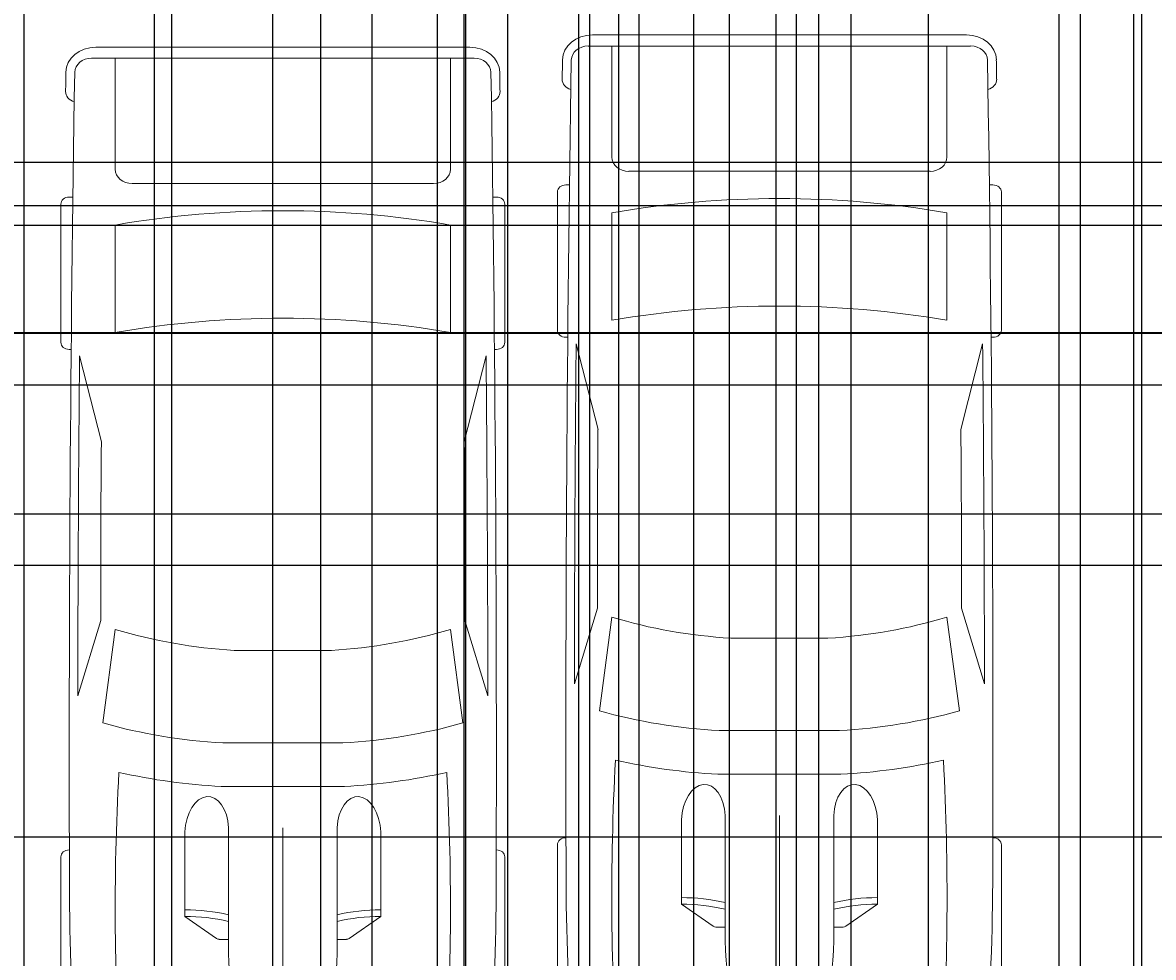
# Model space of a CAD drawing. Units: inches. Extents: x 818 to 1898, y 976 to 2364.
# Tile 19 of 96: x 1207 to 1405, y 1277 to 1441. Entities that reach past the tile are written whole.
import ezdxf

# ---------------------------------------------------------------- set-up
doc = ezdxf.new("R2010")
doc.units = ezdxf.units.IN
doc.header["$LTSCALE"] = 5
doc.header["$MEASUREMENT"] = 0
doc.layers.add('A-ANNO-DIMS', color=2, linetype='Continuous', lineweight=18)
doc.layers.add('C-PKNG', color=8, linetype='Continuous', lineweight=18)
doc.styles.get("Standard").update_dxf_attribs({"font": 'arial.ttf'})
doc.dimstyles.get("Standard").update_dxf_attribs({"dimtxt": 0.18, "dimasz": 0.18, "dimexe": 0.18, "dimexo": 0.0625, "dimgap": 0.09, "dimtad": 0, "dimtih": 1, "dimtoh": 1, "dimdec": 4, "dimzin": 0, "dimdsep": 46, "dimtxsty": 'Standard', "dimcen": 0.09, "dimadec": 0, "dimazin": 0, "dimtfac": 1, "dimtdec": 4, "dimtofl": 0, "dimtmove": 0, "dimatfit": 3, "dimfxl": 1, "dimtolj": 1, "dimtzin": 0, "dimarcsym": 0})

# ---------------------------------------------------------------- blocks, each defined once
blk = doc.blocks.new('*U13')
for p, q in [((46.55, 38.89), (22.35, 38.89)), ((136.7, 38.89), (160.9, 38.89)), ((47.8, 37.39), (47.8, 37.41)), ((87.99, 31.87), (74.76, 35.92)), ((135.45, 37.07), (135.45, 37.41)), ((162.15, 37.41), (162.15, 36.77)), ((134.31, 35.6), (119.29, 31.78)), ((186.47, -33.5), (186.47, 33.5)), ((188.4, -32.76), (188.4, 32.76)), ((70.03, 31.54), (86.41, 29.35)), ((138.42, 29.35), (157.25, 29.35)), ((186.47, 29.35), (167.01, 29.35)), ((164.52, 26.39), (164.52, -26.39)), ((32.27, 11.63), (36.13, 17.17)), ((36.13, 17.17), (50.94, 17.17)), ((32.12, 9.51), (32.12, 11.15)), ((58.92, -10.77), (58.92, 10.77)), ((66.55, -10.53), (66.55, 10.53)), ((186.47, -10.53), (186.47, 10.53)), ((29.77, 9.51), (51.68, 9.51)), ((82.74, 8.5), (82.74, -8.5)), ((0, 0), (51.68, 0)), ((29.77, -9.51), (51.68, -9.51)), ((32.12, -9.51), (32.12, -11.15)), ((32.27, -11.63), (36.13, -17.17)), ((36.13, -17.17), (50.94, -17.17)), ((86.41, -29.35), (70.03, -31.54)), ((157.25, -29.35), (138.42, -29.35)), ((167.01, -29.35), (186.47, -29.35)), ((87.99, -31.87), (74.76, -35.92)), ((134.31, -35.6), (119.29, -31.78)), ((47.8, -37.39), (47.8, -37.41)), ((135.45, -37.07), (135.45, -37.41)), ((162.15, -37.41), (162.15, -36.77)), ((46.55, -38.89), (22.35, -38.89)), ((136.7, -38.89), (160.9, -38.89))]:
    blk.add_line(p, q)
for centre, major_axis, ratio, start_param, end_param in [((46.55, 37.41), (0, 1.48), 0.842304, -1.570796, 0), ((136.7, 37.41), (0, -1.48), 0.842304, 3.141593, 4.712389), ((160.9, 37.41), (0, 1.48), 0.842304, -1.570796, 0), ((180.63, 35.84), (0, 2.22), 0.842304, -0.013017, 1.249894), ((64.48, -10556.36), (0, 10595.31), 0.842304, -0.013397, -0.013017), ((183.98, 32.76), (0, -5.25), 0.842304, 1.570796, 3.128196), ((41.19, -490.86), (0, 528.23), 0.842304, 0.00281, 0.075598), ((64.48, -10555.62), (0, 10593.03), 0.842304, -0.013397, 0.002797), ((64.48, -10555.62), (0, -10591.55), 0.842304, 3.133765, 3.140441), ((183.98, 33.5), (0, -2.96), 0.842304, 1.570796, 3.128196), ((95.79, -3666.35), (0, -3698.24), 0.842304, 3.134049, 3.144098), ((135.29, 5.39), (0, 81.77), 0.842304, 1.245306, 1.50788), ((37.47, -593.96), (0, -623.33), 0.842304, 3.096046, 3.200911), ((134.4, 5.39), (0, -89.78), 0.842304, 4.449482, 4.652344), ((149.6, 2.8), (0, -79.58), 0.842304, 4.372215, 4.640744), ((17.08, 0), (0, 147.02), 0.842304, 4.511394, 4.913384), ((35.91, 0), (0, 147.02), 0.842304, 4.511394, 4.913384), ((167.01, 26.39), (0, 2.96), 0.842304, 0, 1.570796), ((13.04, 17.01), (0, 27.42), 0.842304, 4.435146, 4.718221), ((14.2, 17.01), (0, 27.42), 0.842304, 4.435146, 4.718221), ((50.79, 13.34), (6.34, -0.36), 0.603834, -1.395552, 1.581315), ((32.75, 11.15), (0, 0.74), 0.842304, 0.879714, 1.570796), ((29.77, -46.66), (0, 56.17), 0.842304, 0, 0.590319), ((29.77, 46.66), (0, 56.17), 0.842304, 2.551274, 3.141593), ((13.04, -17.01), (0, -27.42), 0.842304, 1.564964, 1.848039), ((14.2, -17.01), (0, -27.42), 0.842304, 1.564964, 1.848039), ((149.6, -2.8), (0, -79.58), 0.842304, -1.499151, -1.230623), ((32.75, -11.15), (0, -0.74), 0.842304, 4.712389, 5.403472), ((134.4, -5.39), (0, -89.78), 0.842304, -1.510751, -1.307889), ((135.29, -5.39), (0, -81.77), 0.842304, -1.50788, -1.245306), ((167.01, -26.39), (0, -2.96), 0.842304, 4.712389, 6.283185), ((37.47, 593.96), (0, -623.33), 0.842304, -0.059319, 0.045547), ((95.79, 3666.35), (0, -3698.24), 0.842304, -0.002505, 0.007544), ((183.98, -33.5), (0, 2.96), 0.842304, 3.15499, 4.712389), ((183.98, -32.76), (0, -5.25), 0.842304, 0.013397, 1.570796), ((64.48, 10555.62), (0, -10591.55), 0.842304, 0.001152, 0.007828), ((41.19, 490.86), (0, -528.23), 0.842304, -0.075598, -0.00281), ((64.48, 10555.62), (0, 10593.03), 0.842304, 3.138796, 3.15499), ((46.55, -37.41), (0, -1.48), 0.842304, 0, 1.570796), ((136.7, -37.41), (0, -1.48), 0.842304, -1.570796, 0), ((160.9, -37.41), (0, 1.48), 0.842304, 3.141593, 4.712389), ((180.63, -35.84), (0, -2.22), 0.842304, -1.249894, 0.013017), ((64.48, 10556.36), (0, 10595.31), 0.842304, 3.15461, 3.15499)]:
    blk.add_ellipse(centre, major_axis=major_axis, ratio=ratio, start_param=start_param, end_param=end_param)
at = {"extrusion": (0, 0, -1)}
blk.add_ellipse((50.79, -13.34), major_axis=(6.34, 0.36), ratio=0.603834, start_param=-1.395552, end_param=1.581315, dxfattribs=at)
blk = doc.blocks.new('*D59')
at = {"layer": 'A-ANNO-DIMS', "color": 0, "lineweight": -2, "ltscale": 5, "transparency": 16777216}
for p, q in [((1251.64, 2300.39), (818.03, 2300.39)), ((818.21, 2300.21), (818.21, 1669.95)), ((818.21, 1039.32), (818.21, 1669.59)), ((896.05, 1039.14), (818.03, 1039.14))]:
    blk.add_line(p, q, dxfattribs=at)
at = {"layer": 'A-ANNO-DIMS', "color": 0, "ltscale": 5, "transparency": 16777216}
for points in [[(818.18, 2300.21), (818.24, 2300.21), (818.21, 2300.39)], [(818.18, 1039.32), (818.24, 1039.32), (818.21, 1039.14)]]:
    blk.add_solid(points, dxfattribs=at)
at = {"layer": 'Defpoints', "color": 0, "ltscale": 5, "transparency": 16777216}
for p in [(818.21, 2300.39), (1251.71, 2300.39), (896.11, 1039.14)]:
    blk.add_point(p, dxfattribs=at)
at = {"layer": 'A-ANNO-DIMS', "color": 0, "ltscale": 5, "transparency": 16777216, "insert": (818.21, 1669.77), "char_height": 0.18, "attachment_point": 5}
blk.add_mtext('\\A1;1261.2', dxfattribs=at)
blk = doc.blocks.new('*D61')
at = {"layer": 'A-ANNO-DIMS', "color": 0, "lineweight": -2, "ltscale": 5, "transparency": 16777216}
for p, q in [((1071.73, 1203.03), (1071.73, 2363.87)), ((1071.91, 2363.69), (1250.94, 2363.69)), ((1430.55, 2363.69), (1251.51, 2363.69)), ((1430.73, 1203.03), (1430.73, 2363.87))]:
    blk.add_line(p, q, dxfattribs=at)
at = {"layer": 'A-ANNO-DIMS', "color": 0, "ltscale": 5, "transparency": 16777216}
for points in [[(1071.91, 2363.72), (1071.91, 2363.66), (1071.73, 2363.69)], [(1430.55, 2363.72), (1430.55, 2363.66), (1430.73, 2363.69)]]:
    blk.add_solid(points, dxfattribs=at)
at = {"layer": 'Defpoints', "color": 0, "ltscale": 5, "transparency": 16777216}
for p in [(1430.73, 2363.69), (1071.73, 1202.96), (1430.73, 1202.96)]:
    blk.add_point(p, dxfattribs=at)
at = {"layer": 'A-ANNO-DIMS', "color": 0, "ltscale": 5, "transparency": 16777216, "insert": (1251.23, 2363.69), "char_height": 0.18, "attachment_point": 5}
blk.add_mtext('\\A1;359', dxfattribs=at)
blk = doc.blocks.new('*D95')
at = {"layer": 'A-ANNO-DIMS', "color": 0, "lineweight": -2, "ltscale": 5, "transparency": 16777216}
for p, q in [((1173.54, 1071.12), (1173.54, 2363.87)), ((1173.72, 2363.69), (1201.29, 2363.69)), ((1229.47, 2363.69), (1201.9, 2363.69)), ((1229.65, 1071.12), (1229.65, 2363.87))]:
    blk.add_line(p, q, dxfattribs=at)
at = {"layer": 'A-ANNO-DIMS', "color": 0, "ltscale": 5, "transparency": 16777216}
for points in [[(1173.72, 2363.72), (1173.72, 2363.66), (1173.54, 2363.69)], [(1229.47, 2363.72), (1229.47, 2363.66), (1229.65, 2363.69)]]:
    blk.add_solid(points, dxfattribs=at)
at = {"layer": 'Defpoints', "color": 0, "ltscale": 5, "transparency": 16777216}
for p in [(1229.65, 2363.69), (1173.54, 1071.06), (1229.65, 1071.06)]:
    blk.add_point(p, dxfattribs=at)
at = {"layer": 'A-ANNO-DIMS', "color": 0, "ltscale": 5, "transparency": 16777216, "insert": (1201.59, 2363.69), "char_height": 0.18, "attachment_point": 5}
blk.add_mtext('\\A1;56.1', dxfattribs=at)
blk = doc.blocks.new('*D96')
at = {"layer": 'A-ANNO-DIMS', "color": 0, "lineweight": -2, "ltscale": 5, "transparency": 16777216}
for p, q in [((1229.65, 1071.12), (1229.65, 2363.87)), ((1229.83, 2363.69), (1256.52, 2363.69)), ((1283.99, 2363.69), (1257.3, 2363.69)), ((1284.17, 1071.12), (1284.17, 2363.87))]:
    blk.add_line(p, q, dxfattribs=at)
at = {"layer": 'A-ANNO-DIMS', "color": 0, "ltscale": 5, "transparency": 16777216}
for points in [[(1229.83, 2363.72), (1229.83, 2363.66), (1229.65, 2363.69)], [(1283.99, 2363.72), (1283.99, 2363.66), (1284.17, 2363.69)]]:
    blk.add_solid(points, dxfattribs=at)
at = {"layer": 'Defpoints', "color": 0, "ltscale": 5, "transparency": 16777216}
for p in [(1284.17, 2363.69), (1229.65, 1071.06), (1284.17, 1071.06)]:
    blk.add_point(p, dxfattribs=at)
at = {"layer": 'A-ANNO-DIMS', "color": 0, "ltscale": 5, "transparency": 16777216, "insert": (1256.91, 2363.69), "char_height": 0.18, "attachment_point": 5}
blk.add_mtext('\\A1;54.52', dxfattribs=at)
blk = doc.blocks.new('*D97')
at = {"layer": 'A-ANNO-DIMS', "color": 0, "lineweight": -2, "ltscale": 5, "transparency": 16777216}
for p, q in [((1284.17, 1071.12), (1284.17, 2363.87)), ((1284.35, 2363.69), (1310.96, 2363.69)), ((1338.36, 2363.69), (1311.75, 2363.69)), ((1338.54, 1071.12), (1338.54, 2363.87))]:
    blk.add_line(p, q, dxfattribs=at)
at = {"layer": 'A-ANNO-DIMS', "color": 0, "ltscale": 5, "transparency": 16777216}
for points in [[(1284.35, 2363.72), (1284.35, 2363.66), (1284.17, 2363.69)], [(1338.36, 2363.72), (1338.36, 2363.66), (1338.54, 2363.69)]]:
    blk.add_solid(points, dxfattribs=at)
at = {"layer": 'Defpoints', "color": 0, "ltscale": 5, "transparency": 16777216}
for p in [(1338.54, 2363.69), (1284.17, 1071.06), (1338.54, 1071.06)]:
    blk.add_point(p, dxfattribs=at)
at = {"layer": 'A-ANNO-DIMS', "color": 0, "ltscale": 5, "transparency": 16777216, "insert": (1311.36, 2363.69), "char_height": 0.18, "attachment_point": 5}
blk.add_mtext('\\A1;54.37', dxfattribs=at)
blk = doc.blocks.new('*D98')
at = {"layer": 'A-ANNO-DIMS', "color": 0, "lineweight": -2, "ltscale": 5, "transparency": 16777216}
for p, q in [((1338.54, 1071.12), (1338.54, 2363.87)), ((1338.72, 2363.69), (1364.81, 2363.69)), ((1391.7, 2363.69), (1365.6, 2363.69)), ((1391.88, 1071.12), (1391.88, 2363.87))]:
    blk.add_line(p, q, dxfattribs=at)
at = {"layer": 'A-ANNO-DIMS', "color": 0, "ltscale": 5, "transparency": 16777216}
for points in [[(1338.72, 2363.72), (1338.72, 2363.66), (1338.54, 2363.69)], [(1391.7, 2363.72), (1391.7, 2363.66), (1391.88, 2363.69)]]:
    blk.add_solid(points, dxfattribs=at)
at = {"layer": 'Defpoints', "color": 0, "ltscale": 5, "transparency": 16777216}
for p in [(1391.88, 2363.69), (1338.54, 1071.06), (1391.88, 1071.06)]:
    blk.add_point(p, dxfattribs=at)
at = {"layer": 'A-ANNO-DIMS', "color": 0, "ltscale": 5, "transparency": 16777216, "insert": (1365.21, 2363.69), "char_height": 0.18, "attachment_point": 5}
blk.add_mtext('\\A1;53.33', dxfattribs=at)
blk = doc.blocks.new('*D99')
at = {"layer": 'A-ANNO-DIMS', "color": 0, "lineweight": -2, "ltscale": 5, "transparency": 16777216}
for p, q in [((1391.88, 1071.12), (1391.88, 2363.87)), ((1392.06, 2363.69), (1420.45, 2363.69)), ((1449.64, 2363.69), (1421.24, 2363.69)), ((1449.82, 1071.12), (1449.82, 2363.87))]:
    blk.add_line(p, q, dxfattribs=at)
at = {"layer": 'A-ANNO-DIMS', "color": 0, "ltscale": 5, "transparency": 16777216}
for points in [[(1392.06, 2363.72), (1392.06, 2363.66), (1391.88, 2363.69)], [(1449.64, 2363.72), (1449.64, 2363.66), (1449.82, 2363.69)]]:
    blk.add_solid(points, dxfattribs=at)
at = {"layer": 'Defpoints', "color": 0, "ltscale": 5, "transparency": 16777216}
for p in [(1449.82, 2363.69), (1391.88, 1071.06), (1449.82, 1071.06)]:
    blk.add_point(p, dxfattribs=at)
at = {"layer": 'A-ANNO-DIMS', "color": 0, "ltscale": 5, "transparency": 16777216, "insert": (1420.85, 2363.69), "char_height": 0.18, "attachment_point": 5}
blk.add_mtext('\\A1;57.94', dxfattribs=at)
blk = doc.blocks.new('*D112')
at = {"layer": 'A-ANNO-DIMS', "color": 0, "lineweight": -2, "ltscale": 5, "transparency": 16777216}
for p, q in [((1135.27, 1405.71), (1897.92, 1405.71)), ((1897.74, 1405.53), (1897.74, 1396.48)), ((1897.74, 1387.07), (1897.74, 1396.12)), ((1135.27, 1386.89), (1897.92, 1386.89))]:
    blk.add_line(p, q, dxfattribs=at)
at = {"layer": 'A-ANNO-DIMS', "color": 0, "ltscale": 5, "transparency": 16777216}
for points in [[(1897.71, 1405.53), (1897.77, 1405.53), (1897.74, 1405.71)], [(1897.71, 1387.07), (1897.77, 1387.07), (1897.74, 1386.89)]]:
    blk.add_solid(points, dxfattribs=at)
at = {"layer": 'Defpoints', "color": 0, "ltscale": 5, "transparency": 16777216}
for p in [(1135.21, 1405.71), (1135.21, 1386.89), (1897.74, 1386.89)]:
    blk.add_point(p, dxfattribs=at)
at = {"layer": 'A-ANNO-DIMS', "color": 0, "ltscale": 5, "transparency": 16777216, "insert": (1897.74, 1396.3), "char_height": 0.18, "attachment_point": 5}
blk.add_mtext('\\A1;18.824', dxfattribs=at)
blk = doc.blocks.new('*D115')
at = {"layer": 'A-ANNO-DIMS', "color": 0, "lineweight": -2, "ltscale": 5, "transparency": 16777216}
for p, q in [((1766.29, 1377.66), (818.03, 1377.66)), ((818.21, 1377.48), (818.21, 1338.26)), ((818.21, 1298.68), (818.21, 1337.9)), ((1766.29, 1298.5), (818.03, 1298.5))]:
    blk.add_line(p, q, dxfattribs=at)
at = {"layer": 'A-ANNO-DIMS', "color": 0, "ltscale": 5, "transparency": 16777216}
for points in [[(818.18, 1377.48), (818.24, 1377.48), (818.21, 1377.66)], [(818.18, 1298.68), (818.24, 1298.68), (818.21, 1298.5)]]:
    blk.add_solid(points, dxfattribs=at)
at = {"layer": 'Defpoints', "color": 0, "ltscale": 5, "transparency": 16777216}
for p in [(818.21, 1377.66), (1766.35, 1377.66), (1766.35, 1298.5)]:
    blk.add_point(p, dxfattribs=at)
at = {"layer": 'A-ANNO-DIMS', "color": 0, "ltscale": 5, "transparency": 16777216, "insert": (818.21, 1338.08), "char_height": 0.18, "attachment_point": 5}
blk.add_mtext('\\A1;79.15', dxfattribs=at)
blk = doc.blocks.new('*D116')
at = {"layer": 'A-ANNO-DIMS', "color": 0, "lineweight": -2, "ltscale": 5, "transparency": 16777216}
for p, q in [((1766.29, 1456.81), (818.03, 1456.81)), ((818.21, 1456.63), (818.21, 1417.41)), ((818.21, 1377.84), (818.21, 1417.05)), ((1766.29, 1377.66), (818.03, 1377.66))]:
    blk.add_line(p, q, dxfattribs=at)
at = {"layer": 'A-ANNO-DIMS', "color": 0, "ltscale": 5, "transparency": 16777216}
for points in [[(818.18, 1456.63), (818.24, 1456.63), (818.21, 1456.81)], [(818.18, 1377.84), (818.24, 1377.84), (818.21, 1377.66)]]:
    blk.add_solid(points, dxfattribs=at)
at = {"layer": 'Defpoints', "color": 0, "ltscale": 5, "transparency": 16777216}
for p in [(818.21, 1456.81), (1766.35, 1456.81), (1766.35, 1377.66)]:
    blk.add_point(p, dxfattribs=at)
at = {"layer": 'A-ANNO-DIMS', "color": 0, "ltscale": 5, "transparency": 16777216, "insert": (818.21, 1417.23), "char_height": 0.18, "attachment_point": 5}
blk.add_mtext('\\A1;79.15', dxfattribs=at)
blk = doc.blocks.new('*D145')
at = {"layer": 'A-ANNO-DIMS', "color": 0, "lineweight": -2, "ltscale": 5, "transparency": 16777216}
for p, q in [((1197.39, 2122.31), (1197.39, 975.66)), ((1232.61, 2122.31), (1232.61, 975.66)), ((1197.57, 975.84), (1214.61, 975.84)), ((1232.43, 975.84), (1215.39, 975.84))]:
    blk.add_line(p, q, dxfattribs=at)
at = {"layer": 'A-ANNO-DIMS', "color": 0, "ltscale": 5, "transparency": 16777216}
for points in [[(1197.57, 975.87), (1197.57, 975.81), (1197.39, 975.84)], [(1232.43, 975.87), (1232.43, 975.81), (1232.61, 975.84)]]:
    blk.add_solid(points, dxfattribs=at)
at = {"layer": 'Defpoints', "color": 0, "ltscale": 5, "transparency": 16777216}
for p in [(1197.39, 2122.38), (1232.61, 2122.38), (1232.61, 975.84)]:
    blk.add_point(p, dxfattribs=at)
at = {"layer": 'A-ANNO-DIMS', "color": 0, "ltscale": 5, "transparency": 16777216, "insert": (1215, 975.84), "char_height": 0.18, "attachment_point": 5}
blk.add_mtext('\\A1;35.22', dxfattribs=at)
blk = doc.blocks.new('*D159')
at = {"layer": 'A-ANNO-DIMS', "color": 0, "lineweight": -2, "ltscale": 5, "transparency": 16777216}
for p, q in [((1206.73, 1687.02), (1206.73, 975.66)), ((1463.73, 1687.02), (1463.73, 975.66)), ((1206.91, 975.84), (1334.93, 975.84)), ((1463.55, 975.84), (1335.52, 975.84))]:
    blk.add_line(p, q, dxfattribs=at)
at = {"layer": 'A-ANNO-DIMS', "color": 0, "ltscale": 5, "transparency": 16777216}
for points in [[(1206.91, 975.87), (1206.91, 975.81), (1206.73, 975.84)], [(1463.55, 975.87), (1463.55, 975.81), (1463.73, 975.84)]]:
    blk.add_solid(points, dxfattribs=at)
at = {"layer": 'Defpoints', "color": 0, "ltscale": 5, "transparency": 16777216}
for p in [(1206.73, 1687.08), (1463.73, 1687.08), (1463.73, 975.84)]:
    blk.add_point(p, dxfattribs=at)
at = {"layer": 'A-ANNO-DIMS', "color": 0, "ltscale": 5, "transparency": 16777216, "insert": (1335.23, 975.84), "char_height": 0.18, "attachment_point": 5}
blk.add_mtext('\\A1;257', dxfattribs=at)
blk = doc.blocks.new('*D163')
at = {"layer": 'A-ANNO-DIMS', "color": 0, "lineweight": -2, "ltscale": 5, "transparency": 16777216}
for p, q in [((1365.15, 1501.02), (1365.15, 975.66)), ((1401.15, 1501.02), (1401.15, 975.66)), ((1365.33, 975.84), (1382.93, 975.84)), ((1400.97, 975.84), (1383.37, 975.84))]:
    blk.add_line(p, q, dxfattribs=at)
at = {"layer": 'A-ANNO-DIMS', "color": 0, "ltscale": 5, "transparency": 16777216}
for points in [[(1365.33, 975.87), (1365.33, 975.81), (1365.15, 975.84)], [(1400.97, 975.87), (1400.97, 975.81), (1401.15, 975.84)]]:
    blk.add_solid(points, dxfattribs=at)
at = {"layer": 'Defpoints', "color": 0, "ltscale": 5, "transparency": 16777216}
for p in [(1365.15, 1501.08), (1401.15, 1501.08), (1401.15, 975.84)]:
    blk.add_point(p, dxfattribs=at)
at = {"layer": 'A-ANNO-DIMS', "color": 0, "ltscale": 5, "transparency": 16777216, "insert": (1383.15, 975.84), "char_height": 0.18, "attachment_point": 5}
blk.add_mtext('\\A1;36', dxfattribs=at)
blk = doc.blocks.new('*D164')
at = {"layer": 'A-ANNO-DIMS', "color": 0, "lineweight": -2, "ltscale": 5, "transparency": 16777216}
for p, q in [((1206.73, 1501.02), (1206.73, 975.66)), ((1283.82, 1501.02), (1283.82, 975.66)), ((1206.91, 975.84), (1244.97, 975.84)), ((1283.64, 975.84), (1245.58, 975.84))]:
    blk.add_line(p, q, dxfattribs=at)
at = {"layer": 'A-ANNO-DIMS', "color": 0, "ltscale": 5, "transparency": 16777216}
for points in [[(1206.91, 975.87), (1206.91, 975.81), (1206.73, 975.84)], [(1283.64, 975.87), (1283.64, 975.81), (1283.82, 975.84)]]:
    blk.add_solid(points, dxfattribs=at)
at = {"layer": 'Defpoints', "color": 0, "ltscale": 5, "transparency": 16777216}
for p in [(1206.73, 1501.08), (1283.82, 1501.08), (1283.82, 975.84)]:
    blk.add_point(p, dxfattribs=at)
at = {"layer": 'A-ANNO-DIMS', "color": 0, "ltscale": 5, "transparency": 16777216, "insert": (1245.27, 975.84), "char_height": 0.18, "attachment_point": 5}
blk.add_mtext('\\A1;77.1', dxfattribs=at)
blk = doc.blocks.new('*D167')
at = {"layer": 'A-ANNO-DIMS', "color": 0, "lineweight": -2, "ltscale": 5, "transparency": 16777216}
for p, q in [((1345.97, 1486.18), (1345.97, 975.66)), ((1430.73, 1486.18), (1430.73, 975.66)), ((1346.15, 975.84), (1387.95, 975.84)), ((1430.55, 975.84), (1388.74, 975.84))]:
    blk.add_line(p, q, dxfattribs=at)
at = {"layer": 'A-ANNO-DIMS', "color": 0, "ltscale": 5, "transparency": 16777216}
for points in [[(1346.15, 975.87), (1346.15, 975.81), (1345.97, 975.84)], [(1430.55, 975.87), (1430.55, 975.81), (1430.73, 975.84)]]:
    blk.add_solid(points, dxfattribs=at)
at = {"layer": 'Defpoints', "color": 0, "ltscale": 5, "transparency": 16777216}
for p in [(1345.97, 1486.24), (1430.73, 1486.24), (1430.73, 975.84)]:
    blk.add_point(p, dxfattribs=at)
at = {"layer": 'A-ANNO-DIMS', "color": 0, "ltscale": 5, "transparency": 16777216, "insert": (1388.35, 975.84), "char_height": 0.18, "attachment_point": 5}
blk.add_mtext('\\A1;84.76', dxfattribs=at)
blk = doc.blocks.new('*D171')
at = {"layer": 'A-ANNO-DIMS', "color": 0, "lineweight": -2, "ltscale": 5, "transparency": 16777216}
for p, q in [((1616.66, 1386.69), (818.03, 1386.69)), ((818.21, 1386.51), (818.21, 1371.06)), ((818.21, 1355.26), (818.21, 1370.7)), ((1616.66, 1355.08), (818.03, 1355.08))]:
    blk.add_line(p, q, dxfattribs=at)
at = {"layer": 'A-ANNO-DIMS', "color": 0, "ltscale": 5, "transparency": 16777216}
for points in [[(818.18, 1386.51), (818.24, 1386.51), (818.21, 1386.69)], [(818.18, 1355.26), (818.24, 1355.26), (818.21, 1355.08)]]:
    blk.add_solid(points, dxfattribs=at)
at = {"layer": 'Defpoints', "color": 0, "ltscale": 5, "transparency": 16777216}
for p in [(818.21, 1386.69), (1616.73, 1386.69), (1616.73, 1355.08)]:
    blk.add_point(p, dxfattribs=at)
at = {"layer": 'A-ANNO-DIMS', "color": 0, "ltscale": 5, "transparency": 16777216, "insert": (818.21, 1370.88), "char_height": 0.18, "attachment_point": 5}
blk.add_mtext('\\A1;31.61', dxfattribs=at)
blk = doc.blocks.new('*D172')
at = {"layer": 'A-ANNO-DIMS', "color": 0, "lineweight": -2, "ltscale": 5, "transparency": 16777216}
for p, q in [((1616.66, 1416.69), (818.03, 1416.69)), ((818.21, 1416.51), (818.21, 1401.87)), ((818.21, 1386.87), (818.21, 1401.5)), ((1616.66, 1386.69), (818.03, 1386.69))]:
    blk.add_line(p, q, dxfattribs=at)
at = {"layer": 'A-ANNO-DIMS', "color": 0, "ltscale": 5, "transparency": 16777216}
for points in [[(818.18, 1416.51), (818.24, 1416.51), (818.21, 1416.69)], [(818.18, 1386.87), (818.24, 1386.87), (818.21, 1386.69)]]:
    blk.add_solid(points, dxfattribs=at)
at = {"layer": 'Defpoints', "color": 0, "ltscale": 5, "transparency": 16777216}
for p in [(818.21, 1416.69), (1616.73, 1416.69), (1616.73, 1386.69)]:
    blk.add_point(p, dxfattribs=at)
at = {"layer": 'A-ANNO-DIMS', "color": 0, "ltscale": 5, "transparency": 16777216, "insert": (818.21, 1401.69), "char_height": 0.18, "attachment_point": 5}
blk.add_mtext('\\A1;30', dxfattribs=at)
blk = doc.blocks.new('*D190')
at = {"layer": 'A-ANNO-DIMS', "color": 0, "lineweight": -2, "ltscale": 5, "transparency": 16777216}
for p, q in [((1430.66, 1409.05), (818.03, 1409.05)), ((818.21, 1408.87), (818.21, 1377.75)), ((818.21, 1346.26), (818.21, 1377.38)), ((1430.66, 1346.08), (818.03, 1346.08))]:
    blk.add_line(p, q, dxfattribs=at)
at = {"layer": 'A-ANNO-DIMS', "color": 0, "ltscale": 5, "transparency": 16777216}
for points in [[(818.18, 1408.87), (818.24, 1408.87), (818.21, 1409.05)], [(818.18, 1346.26), (818.24, 1346.26), (818.21, 1346.08)]]:
    blk.add_solid(points, dxfattribs=at)
at = {"layer": 'Defpoints', "color": 0, "ltscale": 5, "transparency": 16777216}
for p in [(818.21, 1409.05), (1430.73, 1409.05), (1430.73, 1346.08)]:
    blk.add_point(p, dxfattribs=at)
at = {"layer": 'A-ANNO-DIMS', "color": 0, "ltscale": 5, "transparency": 16777216, "insert": (818.21, 1377.57), "char_height": 0.18, "attachment_point": 5}
blk.add_mtext('\\A1;62.97', dxfattribs=at)
blk = doc.blocks.new('*D231')
at = {"layer": 'A-ANNO-DIMS', "color": 0, "lineweight": -2, "ltscale": 5, "transparency": 16777216}
for p, q in [((1303.93, 1952.98), (1303.93, 975.66)), ((1402.52, 1952.98), (1402.52, 975.66)), ((1304.11, 975.84), (1352.83, 975.84)), ((1402.34, 975.84), (1353.62, 975.84))]:
    blk.add_line(p, q, dxfattribs=at)
at = {"layer": 'A-ANNO-DIMS', "color": 0, "ltscale": 5, "transparency": 16777216}
for points in [[(1304.11, 975.87), (1304.11, 975.81), (1303.93, 975.84)], [(1402.34, 975.87), (1402.34, 975.81), (1402.52, 975.84)]]:
    blk.add_solid(points, dxfattribs=at)
at = {"layer": 'Defpoints', "color": 0, "ltscale": 5, "transparency": 16777216}
for p in [(1303.93, 1953.04), (1402.52, 1953.04), (1402.52, 975.84)]:
    blk.add_point(p, dxfattribs=at)
at = {"layer": 'A-ANNO-DIMS', "color": 0, "ltscale": 5, "transparency": 16777216, "insert": (1353.22, 975.84), "char_height": 0.18, "attachment_point": 5}
blk.add_mtext('\\A1;98.59', dxfattribs=at)
blk = doc.blocks.new('*D233')
at = {"layer": 'A-ANNO-DIMS', "color": 0, "lineweight": -2, "ltscale": 5, "transparency": 16777216}
for p, q in [((1267.73, 2044.02), (1267.73, 975.66)), ((1303.93, 2008.33), (1303.93, 975.66)), ((1267.91, 975.84), (1285.36, 975.84)), ((1303.75, 975.84), (1286.29, 975.84))]:
    blk.add_line(p, q, dxfattribs=at)
at = {"layer": 'A-ANNO-DIMS', "color": 0, "ltscale": 5, "transparency": 16777216}
for points in [[(1267.91, 975.87), (1267.91, 975.81), (1267.73, 975.84)], [(1303.75, 975.87), (1303.75, 975.81), (1303.93, 975.84)]]:
    blk.add_solid(points, dxfattribs=at)
at = {"layer": 'Defpoints', "color": 0, "ltscale": 5, "transparency": 16777216}
for p in [(1267.73, 2044.08), (1303.93, 2008.39), (1303.93, 975.84)]:
    blk.add_point(p, dxfattribs=at)
at = {"layer": 'A-ANNO-DIMS', "color": 0, "ltscale": 5, "transparency": 16777216, "insert": (1285.83, 975.84), "char_height": 0.18, "attachment_point": 5}
blk.add_mtext('\\A1;36.206', dxfattribs=at)
blk = doc.blocks.new('*D236')
at = {"layer": 'A-ANNO-DIMS', "color": 0, "lineweight": -2, "ltscale": 5, "transparency": 16777216}
for p, q in [((1310.91, 2026.14), (1310.91, 975.66)), ((1342.04, 2026.14), (1342.04, 975.66)), ((1311.09, 975.84), (1326.08, 975.84)), ((1341.86, 975.84), (1326.87, 975.84))]:
    blk.add_line(p, q, dxfattribs=at)
at = {"layer": 'A-ANNO-DIMS', "color": 0, "ltscale": 5, "transparency": 16777216}
for points in [[(1311.09, 975.87), (1311.09, 975.81), (1310.91, 975.84)], [(1341.86, 975.87), (1341.86, 975.81), (1342.04, 975.84)]]:
    blk.add_solid(points, dxfattribs=at)
at = {"layer": 'Defpoints', "color": 0, "ltscale": 5, "transparency": 16777216}
for p in [(1310.91, 2026.21), (1342.04, 2026.21), (1342.04, 975.84)]:
    blk.add_point(p, dxfattribs=at)
at = {"layer": 'A-ANNO-DIMS', "color": 0, "ltscale": 5, "transparency": 16777216, "insert": (1326.48, 975.84), "char_height": 0.18, "attachment_point": 5}
blk.add_mtext('\\A1;31.14', dxfattribs=at)
blk = doc.blocks.new('*D245')
at = {"layer": 'A-ANNO-DIMS', "color": 0, "lineweight": -2, "ltscale": 5, "transparency": 16777216}
for p, q in [((1291.48, 1599.31), (1291.48, 975.66)), ((1314.49, 1599.31), (1314.49, 975.66)), ((1291.66, 975.84), (1302.61, 975.84)), ((1314.31, 975.84), (1303.36, 975.84))]:
    blk.add_line(p, q, dxfattribs=at)
at = {"layer": 'A-ANNO-DIMS', "color": 0, "ltscale": 5, "transparency": 16777216}
for points in [[(1291.66, 975.87), (1291.66, 975.81), (1291.48, 975.84)], [(1314.31, 975.87), (1314.31, 975.81), (1314.49, 975.84)]]:
    blk.add_solid(points, dxfattribs=at)
at = {"layer": 'Defpoints', "color": 0, "ltscale": 5, "transparency": 16777216}
for p in [(1291.48, 1599.37), (1314.49, 1599.37), (1314.49, 975.84)]:
    blk.add_point(p, dxfattribs=at)
at = {"layer": 'A-ANNO-DIMS', "color": 0, "ltscale": 5, "transparency": 16777216, "insert": (1302.98, 975.84), "char_height": 0.18, "attachment_point": 5}
blk.add_mtext('\\A1;23.01', dxfattribs=at)
blk = doc.blocks.new('*D251')
at = {"layer": 'A-ANNO-DIMS', "color": 0, "lineweight": -2, "ltscale": 5, "transparency": 16777216}
for p, q in [((1250.3, 1878.33), (1250.3, 975.66)), ((1258.73, 1878.33), (1258.73, 975.66)), ((1250.48, 975.84), (1254.12, 975.84)), ((1258.55, 975.84), (1254.91, 975.84))]:
    blk.add_line(p, q, dxfattribs=at)
at = {"layer": 'A-ANNO-DIMS', "color": 0, "ltscale": 5, "transparency": 16777216}
for points in [[(1250.48, 975.87), (1250.48, 975.81), (1250.3, 975.84)], [(1258.55, 975.87), (1258.55, 975.81), (1258.73, 975.84)]]:
    blk.add_solid(points, dxfattribs=at)
at = {"layer": 'Defpoints', "color": 0, "ltscale": 5, "transparency": 16777216}
for p in [(1250.3, 1878.39), (1258.73, 1878.39), (1258.73, 975.84)]:
    blk.add_point(p, dxfattribs=at)
at = {"layer": 'A-ANNO-DIMS', "color": 0, "ltscale": 5, "transparency": 16777216, "insert": (1254.51, 975.84), "char_height": 0.18, "attachment_point": 5}
blk.add_mtext('\\A1;8.422', dxfattribs=at)
blk = doc.blocks.new('*D252')
at = {"layer": 'A-ANNO-DIMS', "color": 0, "lineweight": -2, "ltscale": 5, "transparency": 16777216}
for p, q in [((1330.3, 2053.02), (1330.3, 975.66)), ((1388.03, 2053.02), (1388.03, 975.66)), ((1330.48, 975.84), (1358.77, 975.84)), ((1387.85, 975.84), (1359.56, 975.84))]:
    blk.add_line(p, q, dxfattribs=at)
at = {"layer": 'A-ANNO-DIMS', "color": 0, "ltscale": 5, "transparency": 16777216}
for points in [[(1330.48, 975.87), (1330.48, 975.81), (1330.3, 975.84)], [(1387.85, 975.87), (1387.85, 975.81), (1388.03, 975.84)]]:
    blk.add_solid(points, dxfattribs=at)
at = {"layer": 'Defpoints', "color": 0, "ltscale": 5, "transparency": 16777216}
for p in [(1330.3, 2053.08), (1388.03, 2053.08), (1388.03, 975.84)]:
    blk.add_point(p, dxfattribs=at)
at = {"layer": 'A-ANNO-DIMS', "color": 0, "ltscale": 5, "transparency": 16777216, "insert": (1359.17, 975.84), "char_height": 0.18, "attachment_point": 5}
blk.add_mtext('\\A1;57.73', dxfattribs=at)
blk = doc.blocks.new('*D254')
at = {"layer": 'A-ANNO-DIMS', "color": 0, "lineweight": -2, "ltscale": 5, "transparency": 16777216}
for p, q in [((1267.73, 2044.02), (1267.73, 975.66)), ((1330.3, 2044.02), (1330.3, 975.66)), ((1267.91, 975.84), (1298.62, 975.84)), ((1330.12, 975.84), (1299.41, 975.84))]:
    blk.add_line(p, q, dxfattribs=at)
at = {"layer": 'A-ANNO-DIMS', "color": 0, "ltscale": 5, "transparency": 16777216}
for points in [[(1267.91, 975.87), (1267.91, 975.81), (1267.73, 975.84)], [(1330.12, 975.87), (1330.12, 975.81), (1330.3, 975.84)]]:
    blk.add_solid(points, dxfattribs=at)
at = {"layer": 'Defpoints', "color": 0, "ltscale": 5, "transparency": 16777216}
for p in [(1267.73, 2044.08), (1330.3, 2044.08), (1330.3, 975.84)]:
    blk.add_point(p, dxfattribs=at)
at = {"layer": 'A-ANNO-DIMS', "color": 0, "ltscale": 5, "transparency": 16777216, "insert": (1299.02, 975.84), "char_height": 0.18, "attachment_point": 5}
blk.add_mtext('\\A1;62.58', dxfattribs=at)
blk = doc.blocks.new('*D278')
at = {"layer": 'A-ANNO-DIMS', "color": 0, "lineweight": -2, "ltscale": 5, "transparency": 16777216}
for p, q in [((1324.03, 1700.74), (1324.03, 975.66)), ((1267.73, 1696.02), (1267.73, 975.66)), ((1267.91, 975.84), (1295.5, 975.84)), ((1323.85, 975.84), (1296.26, 975.84))]:
    blk.add_line(p, q, dxfattribs=at)
at = {"layer": 'A-ANNO-DIMS', "color": 0, "ltscale": 5, "transparency": 16777216}
for points in [[(1267.91, 975.87), (1267.91, 975.81), (1267.73, 975.84)], [(1323.85, 975.87), (1323.85, 975.81), (1324.03, 975.84)]]:
    blk.add_solid(points, dxfattribs=at)
at = {"layer": 'Defpoints', "color": 0, "ltscale": 5, "transparency": 16777216}
for p in [(1324.03, 1700.81), (1267.73, 1696.08), (1324.03, 975.84)]:
    blk.add_point(p, dxfattribs=at)
at = {"layer": 'A-ANNO-DIMS', "color": 0, "ltscale": 5, "transparency": 16777216, "insert": (1295.88, 975.84), "char_height": 0.18, "attachment_point": 5}
blk.add_mtext('\\A1;56.31', dxfattribs=at)
blk = doc.blocks.new('*D279')
at = {"layer": 'A-ANNO-DIMS', "color": 0, "lineweight": -2, "ltscale": 5, "transparency": 16777216}
for p, q in [((1279.13, 1713.75), (1279.13, 975.66)), ((1267.73, 1696.02), (1267.73, 975.66)), ((1267.91, 975.84), (1273.11, 975.84)), ((1278.95, 975.84), (1273.74, 975.84))]:
    blk.add_line(p, q, dxfattribs=at)
at = {"layer": 'A-ANNO-DIMS', "color": 0, "ltscale": 5, "transparency": 16777216}
for points in [[(1267.91, 975.87), (1267.91, 975.81), (1267.73, 975.84)], [(1278.95, 975.87), (1278.95, 975.81), (1279.13, 975.84)]]:
    blk.add_solid(points, dxfattribs=at)
at = {"layer": 'Defpoints', "color": 0, "ltscale": 5, "transparency": 16777216}
for p in [(1279.13, 1713.82), (1267.73, 1696.08), (1267.73, 975.84)]:
    blk.add_point(p, dxfattribs=at)
at = {"layer": 'A-ANNO-DIMS', "color": 0, "ltscale": 5, "transparency": 16777216, "insert": (1273.43, 975.84), "char_height": 0.18, "attachment_point": 5}
blk.add_mtext('\\A1;11.4', dxfattribs=at)
blk = doc.blocks.new('*D283')
at = {"layer": 'A-ANNO-DIMS', "color": 0, "lineweight": -2, "ltscale": 5, "transparency": 16777216}
for p, q in [((1351.6, 1761.39), (1351.6, 975.66)), ((1267.73, 1696.02), (1267.73, 975.66)), ((1267.91, 975.84), (1309.27, 975.84)), ((1351.42, 975.84), (1310.06, 975.84))]:
    blk.add_line(p, q, dxfattribs=at)
at = {"layer": 'A-ANNO-DIMS', "color": 0, "ltscale": 5, "transparency": 16777216}
for points in [[(1267.91, 975.87), (1267.91, 975.81), (1267.73, 975.84)], [(1351.42, 975.87), (1351.42, 975.81), (1351.6, 975.84)]]:
    blk.add_solid(points, dxfattribs=at)
at = {"layer": 'Defpoints', "color": 0, "ltscale": 5, "transparency": 16777216}
for p in [(1351.6, 1761.45), (1267.73, 1696.08), (1351.6, 975.84)]:
    blk.add_point(p, dxfattribs=at)
at = {"layer": 'A-ANNO-DIMS', "color": 0, "ltscale": 5, "transparency": 16777216, "insert": (1309.66, 975.84), "char_height": 0.18, "attachment_point": 5}
blk.add_mtext('\\A1;83.87', dxfattribs=at)
blk = doc.blocks.new('*D285')
at = {"layer": 'A-ANNO-DIMS', "color": 0, "lineweight": -2, "ltscale": 5, "transparency": 16777216}
for p, q in [((1305.83, 1830.02), (1305.83, 975.66)), ((1267.73, 1814.9), (1267.73, 975.66)), ((1267.91, 975.84), (1286.47, 975.84)), ((1305.65, 975.84), (1287.08, 975.84))]:
    blk.add_line(p, q, dxfattribs=at)
at = {"layer": 'A-ANNO-DIMS', "color": 0, "ltscale": 5, "transparency": 16777216}
for points in [[(1267.91, 975.87), (1267.91, 975.81), (1267.73, 975.84)], [(1305.65, 975.87), (1305.65, 975.81), (1305.83, 975.84)]]:
    blk.add_solid(points, dxfattribs=at)
at = {"layer": 'Defpoints', "color": 0, "ltscale": 5, "transparency": 16777216}
for p in [(1305.83, 1830.08), (1267.73, 1814.97), (1267.73, 975.84)]:
    blk.add_point(p, dxfattribs=at)
at = {"layer": 'A-ANNO-DIMS', "color": 0, "ltscale": 5, "transparency": 16777216, "insert": (1286.78, 975.84), "char_height": 0.18, "attachment_point": 5}
blk.add_mtext('\\A1;38.1', dxfattribs=at)

msp = doc.modelspace()

# ---------------------------------------------------------------- block references
at = {"layer": 'C-PKNG', "rotation": 90}
for p in [(1339.1074, 1250.5978), (1252.1115, 1248.4622)]:
    msp.add_blockref('*U13', p, dxfattribs=at)

# ---------------------------------------------------------------- dimensions: what is measured, and where the dimension line sits
at = {"layer": 'A-ANNO-DIMS', "ltscale": 5}
for base, p1, p2, override, picture, middle in [((1430.7251, 2363.6929), (1071.7251, 1202.9642), (1430.7251, 1202.9642), {"dimdec": 0, "dimlfac": 1, "dimrnd": 0, "dimzin": 0, "dimdsep": 46, "dimlunit": 2}, '*D61', (1251.2251, 2363.6929)), ((1229.6474, 2363.6929), (1173.5418, 1071.0552), (1229.6474, 1071.0552), {"dimdec": 1, "dimlfac": 1, "dimrnd": 0, "dimzin": 0, "dimdsep": 46, "dimlunit": 2}, '*D95', (1201.5946, 2363.6929)), ((1284.1697, 2363.6929), (1229.6474, 1071.0552), (1284.1697, 1071.0552), {"dimdec": 2, "dimlfac": 1, "dimrnd": 0, "dimzin": 0, "dimdsep": 46, "dimlunit": 2}, '*D96', (1256.9085, 2363.6929)), ((1338.5412, 2363.6929), (1284.1697, 1071.0552), (1338.5412, 1071.0552), {"dimdec": 2, "dimlfac": 1, "dimrnd": 0, "dimzin": 0, "dimdsep": 46, "dimlunit": 2}, '*D97', (1311.3554, 2363.6929)), ((1391.8757, 2363.6929), (1338.5412, 1071.0552), (1391.8757, 1071.0552), {"dimdec": 2, "dimlfac": 1, "dimrnd": 0, "dimzin": 0, "dimdsep": 46, "dimlunit": 2}, '*D98', (1365.2084, 2363.6929)), ((1449.8196, 2363.6929), (1391.8757, 1071.0552), (1449.8196, 1071.0552), {"dimdec": 2, "dimlfac": 1, "dimrnd": 0, "dimzin": 0, "dimdsep": 46, "dimlunit": 2}, '*D99', (1420.8477, 2363.6929)), ((1232.6091, 975.8433), (1197.3925, 2122.3767), (1232.6091, 2122.3767), {"dimdec": 2, "dimlfac": 1, "dimrnd": 0, "dimzin": 0, "dimdsep": 46, "dimlunit": 2}, '*D145', (1215.0008, 975.8433)), ((1388.0315, 975.8433), (1330.305, 2053.0782), (1388.0315, 2053.0782), {"dimdec": 2, "dimlfac": 1, "dimrnd": 0, "dimzin": 0, "dimdsep": 46, "dimlunit": 2}, '*D252', (1359.1682, 975.8433)), ((1303.9314, 975.8433), (1267.7251, 2044.0782), (1303.9314, 2008.3917), {"dimdec": 3, "dimlfac": 1, "dimrnd": 0, "dimzin": 0, "dimdsep": 46, "dimlunit": 2}, '*D233', (1285.8283, 975.8433)), ((1330.305, 975.8433), (1267.7251, 2044.0782), (1330.305, 2044.0782), {"dimdec": 2, "dimlfac": 1, "dimrnd": 0, "dimzin": 0, "dimdsep": 46, "dimlunit": 2}, '*D254', (1299.0151, 975.8433)), ((1342.0448, 975.8433), (1310.9077, 2026.2074), (1342.0448, 2026.2074), {"dimdec": 2, "dimlfac": 1, "dimrnd": 0, "dimzin": 0, "dimdsep": 46, "dimlunit": 2}, '*D236', (1326.4762, 975.8433)), ((1402.518, 975.8433), (1303.9314, 1953.0408), (1402.518, 1953.0408), {"dimdec": 2, "dimlfac": 1, "dimrnd": 0, "dimzin": 0, "dimdsep": 46, "dimlunit": 2}, '*D231', (1353.2247, 975.8433)), ((1258.7251, 975.8433), (1250.3029, 1878.3919), (1258.7251, 1878.3919), {"dimdec": 3, "dimlfac": 1, "dimrnd": 0, "dimzin": 0, "dimdsep": 46, "dimlunit": 2}, '*D251', (1254.514, 975.8433)), ((1267.7251, 975.8433), (1305.8278, 1830.0844), (1267.7251, 1814.9652), {"dimdec": 1, "dimlfac": 1, "dimrnd": 0, "dimzin": 0, "dimdsep": 46, "dimlunit": 2}, '*D285', (1286.7765, 975.8433)), ((1351.5985, 975.8433), (1267.7251, 1696.0782), (1351.5985, 1761.449), {"dimdec": 2, "dimlfac": 1, "dimrnd": 0, "dimzin": 0, "dimdsep": 46, "dimlunit": 2}, '*D283', (1309.6618, 975.8433)), ((1267.7251, 975.8433), (1279.1253, 1713.8174), (1267.7251, 1696.0782), {"dimdec": 1, "dimlfac": 1, "dimrnd": 0, "dimzin": 0, "dimdsep": 46, "dimlunit": 2}, '*D279', (1273.4252, 975.8433)), ((1324.0334, 975.8433), (1267.7251, 1696.0782), (1324.0334, 1700.8059), {"dimdec": 2, "dimlfac": 1, "dimrnd": 0, "dimzin": 0, "dimdsep": 46, "dimlunit": 2}, '*D278', (1295.8793, 975.8433)), ((1463.7251, 975.8433), (1206.7251, 1687.0782), (1463.7251, 1687.0782), {"dimdec": 0, "dimlfac": 1, "dimrnd": 0, "dimzin": 0, "dimdsep": 46, "dimlunit": 2}, '*D159', (1335.2251, 975.8433)), ((1314.4882, 975.8433), (1291.4787, 1599.3725), (1314.4882, 1599.3725), {"dimdec": 2, "dimlfac": 1, "dimrnd": 0, "dimzin": 0, "dimdsep": 46, "dimlunit": 2}, '*D245', (1302.9835, 975.8433)), ((1283.8183, 975.8433), (1206.7251, 1501.0782), (1283.8183, 1501.0782), {"dimdec": 1, "dimlfac": 1, "dimrnd": 0, "dimzin": 0, "dimdsep": 46, "dimlunit": 2}, '*D164', (1245.2717, 975.8433)), ((1401.1463, 975.8433), (1365.1463, 1501.0782), (1401.1463, 1501.0782), {"dimdec": 0, "dimlfac": 1, "dimrnd": 0, "dimzin": 0, "dimdsep": 46, "dimlunit": 2}, '*D163', (1383.1463, 975.8433)), ((1430.7251, 975.8433), (1345.9651, 1486.2383), (1430.7251, 1486.2383), {"dimdec": 2, "dimlfac": 1, "dimrnd": 0, "dimzin": 0, "dimdsep": 46, "dimlunit": 2}, '*D167', (1388.3451, 975.8433))]:
    dim = msp.add_linear_dim(base=base, p1=p1, p2=p2, dimstyle='Standard', override=override, dxfattribs=at)
    dim.commit()
    dim.dimension.update_dxf_attribs({"geometry": picture, "text_midpoint": middle})
for base, p1, p2, override, picture, middle in [((818.2059, 2300.3929), (896.1138, 1039.1433), (1251.7057, 2300.3929), {"dimdec": 1, "dimlfac": 1, "dimrnd": 0, "dimzin": 0, "dimdsep": 46, "dimlunit": 2}, '*D59', (818.2059, 1669.7681)), ((818.2059, 1456.8088), (1766.3524, 1377.6564), (1766.3524, 1456.8088), {"dimdec": 2, "dimlfac": 1, "dimrnd": 0, "dimzin": 0, "dimdsep": 46, "dimlunit": 2}, '*D116', (818.2059, 1417.2326)), ((818.2059, 1416.6857), (1616.7251, 1386.6857), (1616.7251, 1416.6857), {"dimdec": 0, "dimlfac": 1, "dimrnd": 0, "dimzin": 0, "dimdsep": 46, "dimlunit": 2}, '*D172', (818.2059, 1401.6857)), ((818.2059, 1409.0522), (1430.7251, 1346.0782), (1430.7251, 1409.0522), {"dimdec": 2, "dimlfac": 1, "dimrnd": 0, "dimzin": 0, "dimdsep": 46, "dimlunit": 2}, '*D190', (818.2059, 1377.5652)), ((1897.736, 1386.8851), (1135.2058, 1405.7088), (1135.2058, 1386.8851), {"dimdec": 3, "dimlfac": 1, "dimrnd": 0, "dimzin": 0, "dimdsep": 46, "dimlunit": 2}, '*D112', (1897.736, 1396.297)), ((818.2059, 1386.6857), (1616.7251, 1355.0782), (1616.7251, 1386.6857), {"dimdec": 2, "dimlfac": 1, "dimrnd": 0, "dimzin": 0, "dimdsep": 46, "dimlunit": 2}, '*D171', (818.2059, 1370.882)), ((818.2059, 1377.6564), (1766.3524, 1298.5041), (1766.3524, 1377.6564), {"dimdec": 2, "dimlfac": 1, "dimrnd": 0, "dimzin": 0, "dimdsep": 46, "dimlunit": 2}, '*D115', (818.2059, 1338.0803))]:
    dim = msp.add_linear_dim(base=base, p1=p1, p2=p2, angle=90, dimstyle='Standard', override=override, dxfattribs=at)
    dim.commit()
    dim.dimension.update_dxf_attribs({"geometry": picture, "text_midpoint": middle})

doc.saveas('drawing.dxf')
